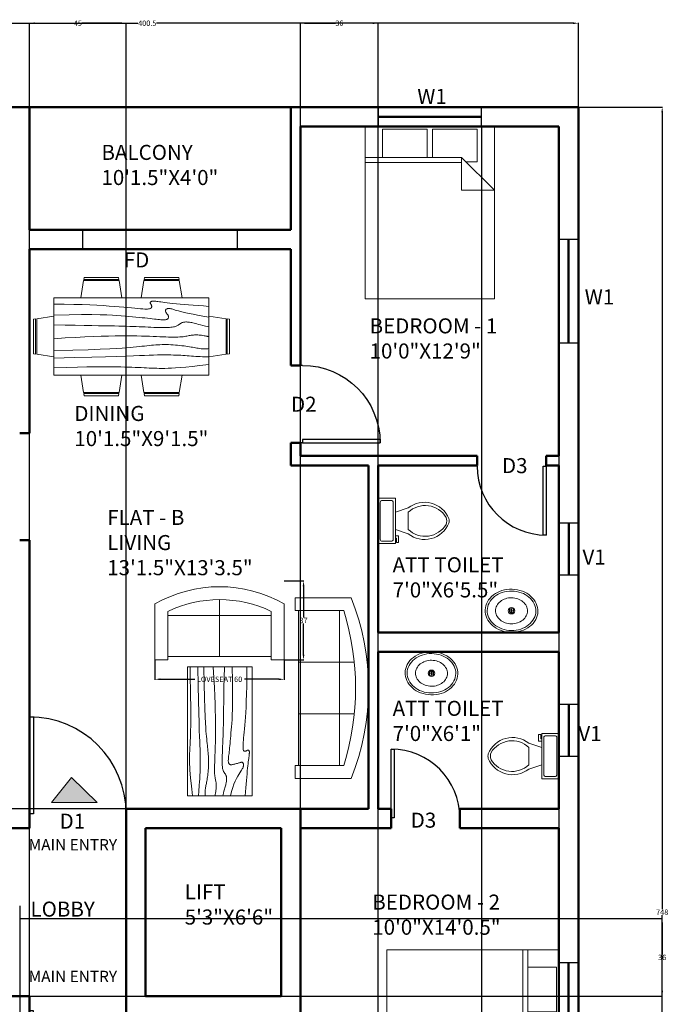
# Model space of a CAD drawing. Units: inches. Extents: x 227 to 711, y 218 to 1048.
# Tile 5 of 5: x 410 to 711, y 590 to 1048. Entities that reach past the tile are written whole.
import ezdxf

# ---------------------------------------------------------------- set-up
doc = ezdxf.new("R2010")
doc.units = ezdxf.units.IN
doc.header["$MEASUREMENT"] = 0
for name, color, linetype, lineweight in [('A-ANNO-DIMS', 2, 'Continuous', 18), ('A-ANNO-SYMB', 85, 'Continuous', 18), ('A-ANNO-TEXT', 70, 'Continuous', 18), ('A-AREA-IDEN', 70, 'Continuous', 25), ('A-FLOR-FIXT', 140, 'Continuous', 18), ('A-FURN', 8, 'Continuous', 18), ('A-WALL', 10, 'Continuous', 50), ('DOORS', 30, 'Continuous', 25), ('WINDOWS', 50, 'Continuous', 25)]:
    doc.layers.add(name, color=color, linetype=linetype, lineweight=lineweight)
doc.styles.get("Standard").update_dxf_attribs({"font": 'arial.ttf'})
doc.dimstyles.get("Standard").update_dxf_attribs({"dimtxt": 2.5, "dimasz": 2.5, "dimexe": 0.18, "dimexo": 0.0625, "dimgap": 0.09, "dimtad": 0, "dimtih": 1, "dimtoh": 1, "dimzin": 0, "dimdsep": 46, "dimlunit": 3, "dimtxsty": 'Standard', "dimcen": 0.09, "dimadec": 0, "dimazin": 0, "dimtfac": 1, "dimtofl": 0, "dimtmove": 0, "dimatfit": 3, "dimfxl": 1, "dimtolj": 1, "dimtzin": 0, "dimarcsym": 0})

# ---------------------------------------------------------------- blocks, each defined once
blk = doc.blocks.new('*U2')
for p, q in [((0, 0), (0, -6)), ((40, 0), (40, -6))]:
    blk.add_line(p, q)
blk.add_lwpolyline([(0, 0), (0, 40), (1.75, 40), (1.75, 0)], close=True)
blk.add_arc((0, 0), 40, 0, 90)
blk = doc.blocks.new('Bed - Queen')
for p, q in [((0, -80.00003), (0, 0)), ((0, 0), (59.99999, 0)), ((59.99999, 0), (59.99999, -80.00003)), ((7.99999, -1.2), (28.79998, -1.2)), ((7.99999, -14.4), (7.99999, -1.2)), ((28.79998, -1.2), (28.79998, -14.4)), ((31.19999, -1.2), (51.99999, -1.2)), ((31.19999, -14.4), (31.19999, -1.2)), ((51.99999, -1.2), (51.99999, -16.4)), ((0, -14.4), (44.8, -14.4)), ((44.8, -16.8), (0, -16.8)), ((59.99999, -29.6), (44.8, -14.4)), ((44.8, -14.4), (44.8, -29.6)), ((51.99999, -16.4), (46.79936, -16.4)), ((44.8, -29.6), (59.99999, -29.6)), ((59.99999, -80.00003), (0, -80.00003))]:
    blk.add_line(p, q)
blk = doc.blocks.new('Toilet - top')
for p, q in [((9.5, -6), (9.5, -2)), ((-10, -8.5), (-8, -8.5)), ((-10, -9.5), (-10, -8.5)), ((-8, -8.5), (-8, -8)), ((-7, -8), (-7, -9.5)), ((-4, -8), (-6, -14)), ((4, -8), (6, -14)), ((-7, -9.5), (-10, -9.5)), ((4, -14), (-4, -14))]:
    blk.add_line(p, q)
blk.add_lwpolyline([(10.5, -8), (10.5, 0), (-10.5, 0), (-10.5, -8)], close=True)
for points in [[(-9.5, -2), (-9.5, -6)], [(8.5, -1), (-8.5, -1)], [(-8.5, -7), (8.5, -7)]]:
    blk.add_lwpolyline(points)
for centre, radius, start, end in [((-8.62, -1.88), 0.884, 81.8699, 188.1301), ((8.62, -1.88), 0.884, 351.8699, 98.1301), ((-8.62, -6.12), 0.884, 171.8699, 278.1301), ((8.62, -6.12), 0.884, 261.8699, 8.1301), ((3.52, -21.58), 12.17, 141.4691, 247.9714), ((4.2, -21.82), 11.33, 136.3677, 238.9468), ((-3.52, -21.58), 12.17, 292.0284, 38.5307), ((-4.2, -21.82), 11.33, 301.053, 43.6321), ((0, -27.88), 4, 245.7318, 294.2682), ((0, -29), 4, 254.8605, 285.1395)]:
    blk.add_arc(centre, radius, start, end)
blk = doc.blocks.new('Sink - Oval top')
for p, q in [((-1, 0), (1, 0)), ((0, 1), (0, -1))]:
    blk.add_line(p, q)
for points in [[(-12.23, 0.39, 0.117634), (-11.46, -3.36, 0.104469), (-8.88, -6.8, 0.090016), (-5.08, -9.07, 0.08192), (-0.32, -10.02, 0.08192), (4.49, -9.38, 0.090016), (8.42, -7.36, 0.104469), (11.22, -4.09, 0.117634), (12.23, -0.39, 0.117634), (11.46, 3.36, 0.104469), (8.88, 6.8, 0.090016), (5.08, 9.07, 0.08192), (0.32, 10.02, 0.08192), (-4.49, 9.38, 0.090016), (-8.42, 7.36, 0.104469), (-11.22, 4.09, 0.117634)], [(-11.29, 0.16, 0.118622), (-10.52, -3.25, 0.104678), (-8.07, -6.36, 0.089562), (-4.54, -8.37, 0.081185), (-0.13, -9.15, 0.081185), (4.3, -8.49, 0.089562), (7.89, -6.58, 0.104678), (10.42, -3.55, 0.118622), (11.29, -0.16, 0.118622), (10.52, 3.25, 0.104678), (8.07, 6.36, 0.089562), (4.54, 8.37, 0.081185), (0.13, 9.15, 0.081185), (-4.3, 8.49, 0.089562), (-7.89, 6.58, 0.104678), (-10.42, 3.55, 0.118622)], [(-7.42, 0.08, 0.118283), (-6.91, -2.17, 0.104607), (-5.29, -4.21, 0.089718), (-2.97, -5.53, 0.081436), (-0.07, -6.04, 0.081436), (2.84, -5.59, 0.089718), (5.2, -4.33, 0.104607), (6.86, -2.32, 0.118283), (7.42, -0.08, 0.118283), (6.91, 2.17, 0.104607), (5.29, 4.21, 0.089718), (2.97, 5.53, 0.081436), (0.07, 6.04, 0.081436), (-2.84, 5.59, 0.089718), (-5.2, 4.33, 0.104607), (-6.86, 2.32, 0.118283)]]:
    blk.add_lwpolyline(points, format="xyb", close=True)
for radius in [1.5, 1]:
    blk.add_circle((0, 0), radius)
blk = doc.blocks.new('Sofa - Roundback 7 ft.')
for p, q in [((-12.00002, -32.4421), (-12.00003, -6.5971)), ((11.99997, -32.4421), (11.99998, -6.5971)), ((-36.000027, -34), (-36.000027, -11.4696)), ((-35.999844, -13.3819), (35.9998, -13.3819)), ((35.99998, -34), (35.99998, -11.4696)), ((-36.000027, -32.4421), (35.99998, -32.4421))]:
    blk.add_line(p, q)
for points in [[(-36.000027, -34), (-42.000027, -34), (-42.000027, -8)], [(41.99998, -8), (41.99998, -34), (35.99998, -34)]]:
    blk.add_lwpolyline(points)
for centre, radius, start, end in [((0, -114.25), 114.25, 68.43141, 111.5686), ((-0.00001, -127.1968), 121.1968, 72.72033, 107.2797)]:
    blk.add_arc(centre, radius, start, end)
blk = doc.blocks.new('Sofa - Roundback Loveseat 5 ft.')
for p, q in [((0, -32.44198), (0, -5.99998)), ((-24, -33.99998), (-24, -11.46958)), ((-23.9998, -13.38178), (23.99986, -13.38178)), ((24.00004, -33.99998), (24.00004, -11.46958)), ((-24, -32.44198), (24.00004, -32.44198))]:
    blk.add_line(p, q)
for points in [[(-24, -33.99998), (-30, -33.99998), (-30, -7.99998)], [(30.00004, -7.99998), (30.00004, -33.99998), (24.00004, -33.99998)]]:
    blk.add_lwpolyline(points)
for centre, radius, start, end in [((0, -60.24998), 60.24998, 60.13715, 119.8628), ((0, -61.38438), 55.38444, 64.32083, 115.6792)]:
    blk.add_arc(centre, radius, start, end)
blk = doc.blocks.new('Dining Set - 36 x 72 in.')
for p, q in [((-22, 27.5), (-22.1562, 26.50042)), ((-22, 27.5), (-6, 27.5)), ((-5.8437, 26.49966), (-6, 27.5)), ((6, 27.5), (5.8438, 26.50042)), ((6, 27.5), (22, 27.5)), ((22.1563, 26.49966), (22, 27.5)), ((-22.2343, 26.00059), (-23.4847, 17.99762)), ((-22.2304, 26), (-5.7608, 26)), ((-5.8416, 26.5), (-22.1534, 26.5)), ((-4.5152, 17.99762), (-5.7655, 25.99926)), ((5.7657, 26.00059), (4.5153, 17.99762)), ((5.7696, 26), (22.2392, 26)), ((22.1584, 26.5), (5.8466, 26.5)), ((23.4848, 17.99762), (22.2345, 25.99926)), ((36, 18), (-36, 18)), ((-36, 18), (-36, -18)), ((36, -18), (36, 18)), ((-44.0006, 8.23428), (-35.9976, 9.48474)), ((44.0006, 8.23428), (35.9976, 9.48474)), ((-45.5, 8), (-44.5004, 8.15617)), ((-45.5, 8), (-45.5, -8)), ((-44.5, -8.15843), (-44.5, 8.15338)), ((-44, 8.23041), (-44, -8.23915)), ((44, 8.23041), (44, -8.23915)), ((44.5, -8.15843), (44.5, 8.15338)), ((45.5, 8), (44.5005, 8.15617)), ((45.5, 8), (45.5, -8)), ((-44.4997, -8.15631), (-45.5, -8)), ((-35.9976, -9.48476), (-43.9993, -8.2345)), ((35.9976, -9.48476), (43.9993, -8.2345)), ((44.4997, -8.15631), (45.5, -8)), ((-36, -18), (36, -18)), ((-22.2343, -26.0006), (-23.4847, -17.99762)), ((-4.5152, -17.99762), (-5.7655, -25.99928)), ((5.7657, -26.0006), (4.5153, -17.99762)), ((23.4848, -17.99762), (22.2345, -25.99928)), ((-22.2304, -26), (-5.7608, -26)), ((-22, -27.5), (-22.1562, -26.50044)), ((-5.8416, -26.5), (-22.1534, -26.5)), ((-5.8437, -26.49967), (-6, -27.5)), ((5.7696, -26), (22.2392, -26)), ((6, -27.5), (5.8438, -26.50044)), ((22.1584, -26.5), (5.8466, -26.5)), ((22.1563, -26.49967), (22, -27.5)), ((-22, -27.5), (-6, -27.5)), ((6, -27.5), (22, -27.5))]:
    blk.add_line(p, q)
for points in [[(-36, 15), (-31.1772, 14.97754), (-26.8079, 14.91406), (-22.8538, 14.81543), (-19.276, 14.6875), (-16.0362, 14.53613), (-13.0957, 14.36718), (-10.4159, 14.18652), (-7.9583, 14), (-5.6904, 13.81315), (-3.6035, 13.63021), (-1.6954, 13.45508), (0.0365, 13.29166), (1.5945, 13.14388), (2.9811, 13.01562), (4.1988, 12.9108), (5.25, 12.83333), (6.1393, 12.78613), (6.8802, 12.76823), (7.4883, 12.77767), (7.9792, 12.8125), (8.3685, 12.87077), (8.6719, 12.95052), (8.9049, 13.0498), (9.0833, 13.16666), (9.2205, 13.29899), (9.3216, 13.44401), (9.3895, 13.59879), (9.4271, 13.76041), (9.4373, 13.92594), (9.4232, 14.09245), (9.3875, 14.257), (9.3333, 14.41666), (9.2638, 14.56917), (9.1836, 14.71484), (9.0975, 14.85465), (9.0104, 14.98958), (8.9272, 15.1206), (8.8529, 15.2487), (8.7922, 15.37483), (8.75, 15.5), (8.7305, 15.62467), (8.7344, 15.74739), (8.7617, 15.86621), (8.8125, 15.97916), (8.8867, 16.08431), (8.9844, 16.17968), (9.1055, 16.26334), (9.25, 16.33333), (9.4189, 16.38802), (9.6172, 16.42708), (9.8506, 16.45052), (10.125, 16.45833), (10.4463, 16.45052), (10.8203, 16.42708), (11.2529, 16.38802), (11.75, 16.33333), (12.3184, 16.26318), (12.9694, 16.17838), (13.7151, 16.07991), (14.5677, 15.96875), (15.5395, 15.84586), (16.6426, 15.71224), (17.8893, 15.56884), (19.2917, 15.41666), (20.859, 15.25667), (22.5879, 15.08984), (24.4721, 14.91715), (26.5052, 14.73958), (28.6809, 14.5581), (30.9929, 14.3737), (33.4347, 14.18733), (36, 14)], [(-36, 10), (-28.9766, 10.14274), (-23.1725, 10.20442), (-18.4241, 10.19775), (-14.5677, 10.13541), (-11.4399, 10.03011), (-8.877, 9.89453), (-6.7154, 9.74137), (-4.7917, 9.58333), (-2.9698, 9.43082), (-1.2246, 9.28515), (0.4415, 9.14534), (2.026, 9.01041), (3.5266, 8.87939), (4.9408, 8.7513), (6.266, 8.62516), (7.5, 8.5), (8.6411, 8.37549), (9.6914, 8.2539), (10.6538, 8.13818), (11.5312, 8.03125), (12.3267, 7.93603), (13.043, 7.85547), (13.6831, 7.79248), (14.25, 7.75), (14.7471, 7.7303), (15.1797, 7.73307), (15.5537, 7.75732), (15.875, 7.80208), (16.1494, 7.86637), (16.3828, 7.94922), (16.5811, 8.04964), (16.75, 8.16666), (16.8944, 8.29915), (17.0143, 8.44531), (17.1089, 8.60319), (17.1771, 8.77083), (17.218, 8.94629), (17.2305, 9.1276), (17.2137, 9.31282), (17.1667, 9.5), (17.0895, 9.6875), (16.987, 9.875), (16.8649, 10.0625), (16.7292, 10.25), (16.5856, 10.4375), (16.4401, 10.625), (16.2985, 10.8125), (16.1667, 11), (16.05, 11.18733), (15.9518, 11.3737), (15.8752, 11.5581), (15.8229, 11.73958), (15.798, 11.91715), (15.8034, 12.08984), (15.842, 12.25667), (15.9167, 12.41666), (16.0295, 12.56836), (16.1784, 12.70833), (16.3605, 12.83268), (16.5729, 12.9375), (16.8127, 13.01888), (17.0768, 13.07291), (17.3625, 13.0957), (17.6667, 13.08333), (17.9894, 13.03312), (18.3418, 12.94726), (18.7382, 12.82918), (19.1927, 12.68229), (19.7195, 12.51001), (20.3327, 12.31575), (21.0465, 12.10294), (21.875, 11.875), (22.8357, 11.63354), (23.959, 11.37304), (25.2786, 11.08618), (26.8282, 10.76562), (28.6414, 10.40405), (30.752, 9.99414), (33.1936, 9.52856), (36, 9)], [(-36, 5.5), (-30.7157, 5.3348), (-26.069, 5.20963), (-21.9946, 5.11767), (-18.4271, 5.05208), (-15.3009, 5.00602), (-12.5508, 4.97265), (-10.1112, 4.94515), (-7.9167, 4.91666), (-5.909, 4.88167), (-4.0586, 4.83984), (-2.3429, 4.79215), (-0.7396, 4.73958), (0.7739, 4.6831), (2.22, 4.6237), (3.6213, 4.56233), (5, 4.5), (6.373, 4.43782), (7.7344, 4.3776), (9.0723, 4.32129), (10.375, 4.27083), (11.6309, 4.22819), (12.8281, 4.19531), (13.9551, 4.17415), (15, 4.16666), (15.954, 4.17448), (16.819, 4.19791), (17.6001, 4.23698), (18.3021, 4.29166), (18.9299, 4.36198), (19.4883, 4.44791), (19.9823, 4.54948), (20.4167, 4.66666), (20.7969, 4.79899), (21.1302, 4.94401), (21.4245, 5.09879), (21.6875, 5.26041), (21.9271, 5.42594), (22.1511, 5.59245), (22.3672, 5.757), (22.5834, 5.91666), (22.8065, 6.06868), (23.0404, 6.21093), (23.2879, 6.34147), (23.5521, 6.45833), (23.8358, 6.55957), (24.142, 6.64323), (24.4735, 6.70735), (24.8334, 6.75), (25.2235, 6.76969), (25.642, 6.76692), (26.0858, 6.74267), (26.5521, 6.69791), (27.0379, 6.63362), (27.5404, 6.55078), (28.0565, 6.45036), (28.5834, 6.33333), (29.1242, 6.19987), (29.7071, 6.04687), (30.3661, 5.87044), (31.1354, 5.66666), (32.0493, 5.43164), (33.142, 5.16146), (34.4475, 4.85221), (36, 4.5)], [(-36, -1), (-30.7915, -0.6591), (-26.0195, -0.38216), (-21.6519, -0.16284), (-17.6563, 0.00521), (-14.0005, 0.12833), (-10.6523, 0.21289), (-7.5796, 0.26522), (-4.75, 0.29166), (-2.134, 0.29793), (0.2878, 0.28711), (2.5317, 0.26163), (4.6146, 0.22396), (6.5529, 0.17651), (8.3633, 0.12174), (10.0623, 0.06209), (11.6667, 0), (13.1899, -0.06201), (14.6341, -0.1211), (15.9982, -0.17432), (17.2813, -0.21875), (18.4823, -0.25147), (19.6003, -0.26953), (20.6343, -0.27002), (21.5834, -0.25), (22.4481, -0.20768), (23.2357, -0.14584), (23.9549, -0.06836), (24.6146, 0.02083), (25.2235, 0.11784), (25.7904, 0.21875), (26.3241, 0.31966), (26.8334, 0.41666), (27.3265, 0.50618), (27.8099, 0.58593), (28.2894, 0.65397), (28.7709, 0.70833), (29.2601, 0.74707), (29.763, 0.76823), (30.2855, 0.76985), (30.8334, 0.75), (31.4088, 0.70784), (31.9994, 0.64713), (32.589, 0.57275), (33.1615, 0.48958), (33.7008, 0.4025), (34.1908, 0.3164), (34.6153, 0.23616), (34.9584, 0.16666), (35.2099, 0.11165), (35.3848, 0.07031), (35.504, 0.04069), (35.5886, 0.02083), (35.6594, 0.00879), (35.7377, 0.0026), (35.8442, 0.00032), (36, 0)], [(-36, -6.5), (-27.1843, -6.31267), (-20.084, -6.1263), (-14.469, -5.9419), (-10.1094, -5.76042), (-6.7752, -5.58285), (-4.2363, -5.41016), (-2.2629, -5.24333), (-0.625, -5.08334), (0.8708, -4.93099), (2.2715, -4.78646), (3.5872, -4.64974), (4.8281, -4.52084), (6.0046, -4.39974), (7.127, -4.28646), (8.2053, -4.18099), (9.25, -4.08334), (10.2705, -3.99382), (11.2734, -3.91407), (12.2647, -3.84603), (13.25, -3.79167), (14.2354, -3.75293), (15.2266, -3.73177), (16.2295, -3.73015), (17.25, -3.75), (18.2912, -3.79248), (19.3451, -3.85547), (20.4009, -3.93604), (21.4479, -4.03125), (22.4754, -4.13819), (23.4727, -4.25391), (24.4289, -4.37549), (25.3334, -4.5), (26.1785, -4.62492), (26.9694, -4.74935), (27.7145, -4.87281), (28.4219, -4.99479), (29.1, -5.11483), (29.7572, -5.23242), (30.4016, -5.34709), (31.0417, -5.45834), (31.6837, -5.56437), (32.3262, -5.65821), (32.9658, -5.73153), (33.599, -5.77604), (34.2224, -5.78345), (34.8327, -5.74545), (35.4264, -5.65373), (36, -5.5)], [(-36, -10), (-26.4022, -9.81299), (-18.4675, -9.62891), (-11.9839, -9.45069), (-6.7396, -9.28125), (-2.5226, -9.12354), (0.8789, -8.98047), (3.6769, -8.85498), (6.0833, -8.75), (8.2767, -8.66765), (10.3021, -8.60677), (12.1712, -8.56543), (13.8958, -8.54167), (15.4876, -8.53353), (16.9583, -8.53907), (18.3197, -8.55632), (19.5834, -8.58334), (20.7616, -8.61841), (21.8685, -8.66081), (22.9188, -8.71004), (23.9271, -8.76563), (24.9081, -8.82707), (25.8763, -8.89388), (26.8465, -8.96558), (27.8334, -9.04167), (28.8474, -9.12118), (29.8828, -9.20117), (30.93, -9.27824), (31.9792, -9.34896), (33.0205, -9.40991), (34.0443, -9.45768), (35.0407, -9.48885), (36, -9.5)], [(-36, -14.5), (-30.0881, -14.33513), (-25.0332, -14.21224), (-20.7312, -14.12647), (-17.0781, -14.07292), (-13.97, -14.04671), (-11.3027, -14.04297), (-8.9724, -14.05681), (-6.875, -14.08334), (-4.9224, -14.11833), (-3.0905, -14.16016), (-1.3709, -14.20785), (0.2448, -14.26042), (1.7647, -14.3169), (3.1973, -14.3763), (4.5507, -14.43767), (5.8333, -14.5), (7.0554, -14.5621), (8.235, -14.62175), (9.3922, -14.67652), (10.5469, -14.72396), (11.7192, -14.76164), (12.929, -14.78711), (14.1965, -14.79794), (15.5417, -14.79167), (16.9933, -14.76424), (18.6152, -14.70508), (20.4804, -14.60197), (22.6615, -14.44271), (25.2312, -14.21509), (28.2624, -13.9069), (31.8277, -13.50594), (36, -13)]]:
    blk.add_lwpolyline(points)
blk = doc.blocks.new('Table - Rectangular Woodgrain 60 x 30 in.')
for p, q in [((0, 0), (0, -30)), ((60, 0), (0, 0)), ((60, -30), (60, 0)), ((0, -30), (60, -30))]:
    blk.add_line(p, q)
for points in [[(0, -2.4), (4.8155, -2.418), (9.0302, -2.4688), (12.709, -2.5477), (15.9167, -2.65), (18.7181, -2.7711), (21.1781, -2.9063), (23.3616, -3.0508), (25.3333, -3.2), (27.1477, -3.3495), (28.8172, -3.4958), (30.3437, -3.636), (31.7291, -3.7667), (32.9756, -3.8849), (34.0849, -3.9875), (35.059, -4.0714), (35.9, -4.1334), (36.6114, -4.1711), (37.2041, -4.1854), (37.6906, -4.1779), (38.0833, -4.15), (38.3948, -4.1034), (38.6375, -4.0396), (38.8239, -3.9602), (38.9666, -3.8667), (39.0764, -3.7608), (39.1573, -3.6448), (39.2116, -3.521), (39.2416, -3.3917), (39.2498, -3.2593), (39.2385, -3.1261), (39.21, -2.9944), (39.1666, -2.8667), (39.111, -2.7447), (39.0468, -2.6281), (38.978, -2.5163), (38.9083, -2.4083), (38.8418, -2.3035), (38.7823, -2.201), (38.7337, -2.1001), (38.7, -2), (38.6844, -1.9003), (38.6875, -1.8021), (38.7094, -1.707), (38.75, -1.6167), (38.8094, -1.5326), (38.8875, -1.4563), (38.9844, -1.3893), (39.1, -1.3333), (39.2351, -1.2896), (39.3937, -1.2583), (39.5804, -1.2396), (39.8, -1.2333), (40.057, -1.2396), (40.3562, -1.2583), (40.7023, -1.2896), (41.1, -1.3333), (41.5547, -1.3895), (42.0755, -1.4573), (42.6721, -1.5361), (43.3542, -1.625), (44.1316, -1.7233), (45.014, -1.8302), (46.0114, -1.9449), (47.1333, -2.0667), (48.3862, -2.1947), (49.7625, -2.3281), (51.2513, -2.4663), (52.8416, -2.6083), (54.5226, -2.7535), (56.2833, -2.9011), (58.1127, -3.0501), (60, -3.2)], [(0, -9.2), (6.5759, -9.0858), (11.9385, -9.0365), (16.2527, -9.0418), (19.6833, -9.0917), (22.3952, -9.1759), (24.5531, -9.2844), (26.322, -9.4069), (27.8666, -9.5333), (29.3241, -9.6553), (30.7203, -9.7719), (32.0532, -9.8837), (33.3208, -9.9917), (34.5213, -10.0965), (35.6526, -10.199), (36.7128, -10.2999), (37.7, -10.4), (38.6129, -10.4996), (39.4531, -10.5969), (40.223, -10.6895), (40.925, -10.775), (41.5613, -10.8512), (42.1344, -10.9156), (42.6465, -10.966), (43.1, -11), (43.4976, -11.0158), (43.8437, -11.0136), (44.143, -10.9942), (44.4, -10.9583), (44.6195, -10.9069), (44.8062, -10.8406), (44.9648, -10.7603), (45.1, -10.6667), (45.2155, -10.5598), (45.3114, -10.4365), (45.3871, -10.2929), (45.4416, -10.125), (45.4743, -9.929), (45.4844, -9.7011), (45.4709, -9.4371), (45.4333, -9.1333), (45.3716, -8.7883), (45.2896, -8.4104), (45.1919, -8.0107), (45.0833, -7.6), (44.9685, -7.1893), (44.8521, -6.7896), (44.7388, -6.4117), (44.6333, -6.0667), (44.54, -5.7628), (44.4614, -5.4979), (44.4001, -5.2675), (44.3583, -5.0667), (44.3384, -4.8909), (44.3427, -4.7354), (44.3736, -4.5956), (44.4333, -4.4667), (44.5236, -4.3453), (44.6427, -4.2333), (44.7884, -4.1339), (44.9583, -4.05), (45.1501, -3.9849), (45.3614, -3.9417), (45.59, -3.9234), (45.8333, -3.9333), (46.0915, -3.9749), (46.3734, -4.0531), (46.6906, -4.1736), (47.0542, -4.3417), (47.4756, -4.5629), (47.9661, -4.8427), (48.5372, -5.1866), (49.2, -5.6), (49.9676, -6.0844), (50.8594, -6.625), (51.8965, -7.2031), (53.1, -7.8), (54.491, -8.3969), (56.0906, -8.975), (57.9199, -9.5156), (60, -10)], [(0, -12.8), (5.1847, -12.9322), (9.6213, -13.0323), (13.3963, -13.1059), (16.5958, -13.1583), (19.3063, -13.1952), (21.614, -13.2219), (23.6054, -13.2439), (25.3666, -13.2667), (26.9728, -13.2947), (28.4531, -13.3281), (29.8256, -13.3663), (31.1083, -13.4083), (32.3191, -13.4535), (33.476, -13.501), (34.597, -13.5501), (35.7, -13.6), (36.7984, -13.6497), (37.8875, -13.6979), (38.9578, -13.743), (40, -13.7833), (41.0047, -13.8174), (41.9625, -13.8438), (42.864, -13.8607), (43.7, -13.8667), (44.4631, -13.8604), (45.1552, -13.8417), (45.7801, -13.8104), (46.3416, -13.7667), (46.8439, -13.7104), (47.2906, -13.6417), (47.6858, -13.5604), (48.0333, -13.4667), (48.3375, -13.3608), (48.6042, -13.2448), (48.8396, -13.121), (49.05, -12.9917), (49.2417, -12.8593), (49.4208, -12.7261), (49.5937, -12.5944), (49.7667, -12.4667), (49.9452, -12.3451), (50.1323, -12.2313), (50.3303, -12.1268), (50.5416, -12.0333), (50.7686, -11.9524), (51.0135, -11.8854), (51.2788, -11.8341), (51.5666, -11.8), (51.8785, -11.7843), (52.2116, -11.7865), (52.562, -11.8059), (52.926, -11.8417), (53.2998, -11.8931), (53.6795, -11.9594), (54.0614, -12.0397), (54.4416, -12.1333), (54.8223, -12.2401), (55.2293, -12.3625), (55.6942, -12.5037), (56.2489, -12.6667), (56.9251, -12.8547), (57.7545, -13.0708), (58.7689, -13.3182), (60, -13.6)], [(0, -18), (5.124, -17.7273), (9.6609, -17.5057), (13.6705, -17.3303), (17.2125, -17.1958), (20.3467, -17.0973), (23.1328, -17.0297), (25.6307, -16.9878), (27.9, -16.9667), (29.9928, -16.9617), (31.9302, -16.9703), (33.7254, -16.9907), (35.3917, -17.0208), (36.9423, -17.0588), (38.3906, -17.1026), (39.7499, -17.1503), (41.0333, -17.2), (42.2519, -17.2496), (43.4073, -17.2969), (44.4986, -17.3395), (45.525, -17.375), (46.4858, -17.4012), (47.3802, -17.4156), (48.2074, -17.416), (48.9667, -17.4), (49.6583, -17.3662), (50.2872, -17.3167), (50.8595, -17.2547), (51.3812, -17.1833), (51.8584, -17.1057), (52.2971, -17.025), (52.7034, -16.9443), (53.0833, -16.8667), (53.443, -16.7951), (53.789, -16.7313), (54.128, -16.6768), (54.4666, -16.6334), (54.8115, -16.6024), (55.1693, -16.5854), (55.5465, -16.5841), (55.95, -16.6), (56.3828, -16.6337), (56.8346, -16.6823), (57.2915, -16.7418), (57.7396, -16.8084), (58.165, -16.878), (58.5539, -16.9469), (58.8924, -17.0111), (59.1666, -17.0667), (59.3679, -17.1107), (59.5078, -17.1438), (59.6032, -17.1675), (59.6708, -17.1833), (59.7275, -17.193), (59.7901, -17.1979), (59.8753, -17.1998), (60, -17.2)], [(0, -22.4), (8.0098, -22.2501), (14.4094, -22.1011), (19.4168, -21.9535), (23.25, -21.8083), (26.1269, -21.6663), (28.2656, -21.5281), (29.884, -21.3947), (31.2, -21.2667), (32.3967, -21.1448), (33.5172, -21.0292), (34.5697, -20.9198), (35.5625, -20.8167), (36.5037, -20.7198), (37.4015, -20.6292), (38.2642, -20.5448), (39.1, -20.4667), (39.9164, -20.3951), (40.7187, -20.3313), (41.5117, -20.2768), (42.3, -20.2333), (43.0883, -20.2024), (43.8812, -20.1854), (44.6836, -20.1841), (45.5, -20.2), (46.3328, -20.234), (47.1747, -20.2844), (48.0163, -20.3488), (48.8479, -20.425), (49.66, -20.5106), (50.4429, -20.6031), (51.1872, -20.7004), (51.8833, -20.8), (52.5246, -20.8999), (53.1166, -20.9995), (53.6681, -21.0983), (54.1875, -21.1958), (54.6834, -21.2919), (55.1646, -21.3859), (55.6394, -21.4777), (56.1167, -21.5667), (56.6028, -21.6515), (57.0961, -21.7266), (57.5929, -21.7852), (58.0896, -21.8208), (58.5823, -21.8268), (59.0674, -21.7964), (59.5412, -21.723), (60, -21.6)], [(0, -25.2), (8.6355, -25.0504), (15.7026, -24.9031), (21.4049, -24.7606), (25.9458, -24.625), (29.529, -24.4988), (32.3578, -24.3844), (34.6359, -24.284), (36.5667, -24.2), (38.3213, -24.1341), (39.9417, -24.0854), (41.437, -24.0523), (42.8167, -24.0333), (44.0901, -24.0268), (45.2667, -24.0313), (46.3557, -24.0451), (47.3667, -24.0667), (48.309, -24.0947), (49.1928, -24.1287), (50.0284, -24.168), (50.826, -24.2125), (51.5959, -24.2617), (52.3483, -24.3151), (53.0935, -24.3725), (53.8417, -24.4334), (54.6009, -24.497), (55.3699, -24.561), (56.1454, -24.6226), (56.9239, -24.6792), (57.7021, -24.7279), (58.4764, -24.7662), (59.2435, -24.7911), (60, -24.8)], [(0, -28.8), (5.6867, -28.6681), (10.45, -28.5698), (14.407, -28.5012), (17.675, -28.4584), (20.3711, -28.4374), (22.6125, -28.4344), (24.5164, -28.4455), (26.2, -28.4667), (27.762, -28.4947), (29.2276, -28.5281), (30.6033, -28.5663), (31.8958, -28.6084), (33.1118, -28.6535), (34.2578, -28.7011), (35.3405, -28.7501), (36.3666, -28.8), (37.3443, -28.8497), (38.288, -28.8974), (39.2137, -28.9412), (40.1375, -28.9792), (41.0753, -29.0093), (42.0432, -29.0297), (43.0572, -29.0384), (44.1333, -29.0333), (45.2936, -29.0114), (46.5843, -28.9641), (48.0579, -28.8816), (49.7666, -28.7542), (51.7629, -28.5721), (54.0989, -28.3255), (56.8272, -28.0048), (60, -27.6)]]:
    blk.add_lwpolyline(points)
blk = doc.blocks.new('WIN-48IN')
for p, q in [((0, 4.75), (48, 4.75)), ((0, 4.25), (48, 4.25))]:
    blk.add_line(p, q)
blk.add_lwpolyline([(0, 0), (48, 0), (48, 9), (0, 9)], close=True)
blk = doc.blocks.new('VENT-V1-24IN')
for p, q in [((4.25, 24), (4.25, 0)), ((4.75, 24), (4.75, 0))]:
    blk.add_line(p, q)
blk.add_lwpolyline([(0, 24), (0, 0), (9, 0), (9, 24)], close=True)
blk = doc.blocks.new('DOOR-FD-72IN')
blk.add_lwpolyline([(0, 0), (72, 0), (72, 9), (0, 9)], close=True)
blk = doc.blocks.new('ENTRY-DIRECTION')
h = blk.add_hatch(color=256)
h.dxf.hatch_style = 1
h.paths.add_polyline_path([(21.25, 11.69), (0, 11.44), (12.11, 0)])
for p, q in [((21.25, 11.69), (0, 11.44)), ((0, 11.44), (12.11, 0)), ((12.11, 0), (21.25, 11.69))]:
    blk.add_line(p, q)
blk = doc.blocks.new('*D42')
at = {"layer": 'A-ANNO-DIMS', "color": 0, "lineweight": -2, "transparency": 16777216}
for p, q in [((472.84, 750.2), (472.84, 741.08)), ((532.84, 750.2), (532.84, 741.08)), ((475.34, 741.26), (491.31, 741.26)), ((530.34, 741.26), (514.36, 741.26))]:
    blk.add_line(p, q, dxfattribs=at)
at = {"layer": 'A-ANNO-DIMS', "color": 0, "transparency": 16777216}
for points in [[(475.34, 741.68), (475.34, 740.85), (472.84, 741.26)], [(530.34, 741.68), (530.34, 740.85), (532.84, 741.26)]]:
    blk.add_solid(points, dxfattribs=at)
at = {"layer": 'Defpoints', "color": 0, "transparency": 16777216}
for p in [(472.84, 750.26), (532.84, 750.26), (532.84, 741.26)]:
    blk.add_point(p, dxfattribs=at)
at = {"layer": 'A-ANNO-DIMS', "color": 0, "transparency": 16777216, "insert": (502.84, 741.26), "char_height": 2.5, "attachment_point": 5}
blk.add_mtext('\\A1;LOVESEAT 60', dxfattribs=at)
blk = doc.blocks.new('*D43')
at = {"layer": 'A-ANNO-DIMS', "color": 0, "lineweight": -2, "transparency": 16777216}
for p, q in [((532.9, 786.93), (542.02, 786.93)), ((541.84, 784.43), (541.84, 769.96)), ((541.84, 752.76), (541.84, 767.23)), ((532.9, 750.26), (542.02, 750.26))]:
    blk.add_line(p, q, dxfattribs=at)
at = {"layer": 'A-ANNO-DIMS', "color": 0, "transparency": 16777216}
for points in [[(541.42, 784.43), (542.25, 784.43), (541.84, 786.93)], [(541.42, 752.76), (542.25, 752.76), (541.84, 750.26)]]:
    blk.add_solid(points, dxfattribs=at)
at = {"layer": 'Defpoints', "color": 0, "transparency": 16777216}
for p in [(532.84, 786.93), (541.84, 786.93), (532.84, 750.26)]:
    blk.add_point(p, dxfattribs=at)
at = {"layer": 'A-ANNO-DIMS', "color": 0, "transparency": 16777216, "insert": (541.84, 768.6), "char_height": 2.5, "attachment_point": 5}
blk.add_mtext('\\A1;37', dxfattribs=at)
blk = doc.blocks.new('*D44')
at = {"layer": 'A-ANNO-DIMS', "color": 0, "lineweight": -2, "transparency": 16777216}
for p, q in [((268.99, 1007.13), (268.99, 1046.2)), ((271.49, 1046.02), (464.87, 1046.02)), ((666.99, 1046.02), (473.61, 1046.02)), ((669.49, 1007.13), (669.49, 1046.2))]:
    blk.add_line(p, q, dxfattribs=at)
at = {"layer": 'A-ANNO-DIMS', "color": 0, "transparency": 16777216}
for points in [[(271.49, 1046.43), (271.49, 1045.6), (268.99, 1046.02)], [(666.99, 1046.43), (666.99, 1045.6), (669.49, 1046.02)]]:
    blk.add_solid(points, dxfattribs=at)
at = {"layer": 'Defpoints', "color": 0, "transparency": 16777216}
for p in [(669.49, 1046.02), (268.99, 1007.07), (669.49, 1007.07)]:
    blk.add_point(p, dxfattribs=at)
at = {"layer": 'A-ANNO-DIMS', "color": 0, "transparency": 16777216, "insert": (469.24, 1046.02), "char_height": 2.5, "attachment_point": 5}
blk.add_mtext('\\A1;400.5', dxfattribs=at)
blk = doc.blocks.new('*D45')
at = {"layer": 'A-ANNO-DIMS', "color": 0, "lineweight": -2, "transparency": 16777216}
for p, q in [((669.55, 1007.07), (708.62, 1007.07)), ((708.44, 1004.57), (708.44, 634.43)), ((708.44, 261.57), (708.44, 631.7)), ((669.55, 259.07), (708.62, 259.07))]:
    blk.add_line(p, q, dxfattribs=at)
at = {"layer": 'A-ANNO-DIMS', "color": 0, "transparency": 16777216}
for points in [[(708.02, 1004.57), (708.86, 1004.57), (708.44, 1007.07)], [(708.02, 261.57), (708.86, 261.57), (708.44, 259.07)]]:
    blk.add_solid(points, dxfattribs=at)
at = {"layer": 'Defpoints', "color": 0, "transparency": 16777216}
for p in [(669.49, 1007.07), (708.44, 1007.07), (669.49, 259.07)]:
    blk.add_point(p, dxfattribs=at)
at = {"layer": 'A-ANNO-DIMS', "color": 0, "transparency": 16777216, "insert": (708.44, 633.07), "char_height": 2.5, "attachment_point": 5}
blk.add_mtext('\\A1;748', dxfattribs=at)
blk = doc.blocks.new('*D51')
at = {"layer": 'A-ANNO-DIMS', "color": 0, "lineweight": -2, "transparency": 16777216}
for p, q in [((268.93, 1007.07), (229.86, 1007.07)), ((230.04, 1004.57), (230.04, 845.43)), ((230.04, 683.57), (230.04, 842.7)), ((459.43, 681.07), (229.86, 681.07))]:
    blk.add_line(p, q, dxfattribs=at)
at = {"layer": 'A-ANNO-DIMS', "color": 0, "transparency": 16777216}
for points in [[(229.62, 1004.57), (230.46, 1004.57), (230.04, 1007.07)], [(229.62, 683.57), (230.46, 683.57), (230.04, 681.07)]]:
    blk.add_solid(points, dxfattribs=at)
at = {"layer": 'Defpoints', "color": 0, "transparency": 16777216}
for p in [(230.04, 1007.07), (268.99, 1007.07), (459.49, 681.07)]:
    blk.add_point(p, dxfattribs=at)
at = {"layer": 'A-ANNO-DIMS', "color": 0, "transparency": 16777216, "insert": (230.04, 844.07), "char_height": 2.5, "attachment_point": 5}
blk.add_mtext('\\A1;326', dxfattribs=at)
blk = doc.blocks.new('*D53')
at = {"layer": 'A-ANNO-DIMS', "color": 0, "lineweight": -2, "transparency": 16777216}
for p, q in [((414.49, 585.13), (414.49, 1046.2)), ((416.99, 1046.02), (435.05, 1046.02)), ((456.99, 1046.02), (438.93, 1046.02)), ((459.49, 585.13), (459.49, 1046.2))]:
    blk.add_line(p, q, dxfattribs=at)
at = {"layer": 'A-ANNO-DIMS', "color": 0, "transparency": 16777216}
for points in [[(416.99, 1046.43), (416.99, 1045.6), (414.49, 1046.02)], [(456.99, 1046.43), (456.99, 1045.6), (459.49, 1046.02)]]:
    blk.add_solid(points, dxfattribs=at)
at = {"layer": 'Defpoints', "color": 0, "transparency": 16777216}
for p in [(459.49, 1046.02), (414.49, 585.07), (459.49, 585.07)]:
    blk.add_point(p, dxfattribs=at)
at = {"layer": 'A-ANNO-DIMS', "color": 0, "transparency": 16777216, "insert": (436.99, 1046.02), "char_height": 2.5, "attachment_point": 5}
blk.add_mtext('\\A1;45', dxfattribs=at)
blk = doc.blocks.new('*D56')
at = {"layer": 'A-ANNO-DIMS', "color": 0, "lineweight": -2, "transparency": 16777216}
for p, q in [((540.49, 493.63), (540.49, 1046.2)), ((542.99, 1046.02), (556.61, 1046.02)), ((573.99, 1046.02), (560.37, 1046.02)), ((576.49, 493.03), (576.49, 1046.2))]:
    blk.add_line(p, q, dxfattribs=at)
at = {"layer": 'A-ANNO-DIMS', "color": 0, "transparency": 16777216}
for points in [[(542.99, 1046.43), (542.99, 1045.6), (540.49, 1046.02)], [(573.99, 1046.43), (573.99, 1045.6), (576.49, 1046.02)]]:
    blk.add_solid(points, dxfattribs=at)
at = {"layer": 'Defpoints', "color": 0, "transparency": 16777216}
for p in [(576.49, 1046.02), (540.49, 493.57), (576.49, 492.97)]:
    blk.add_point(p, dxfattribs=at)
at = {"layer": 'A-ANNO-DIMS', "color": 0, "transparency": 16777216, "insert": (558.49, 1046.02), "char_height": 2.5, "attachment_point": 5}
blk.add_mtext('\\A1;36', dxfattribs=at)
blk = doc.blocks.new('*D59')
at = {"layer": 'A-ANNO-DIMS', "color": 0, "lineweight": -2, "transparency": 16777216}
for p, q in [((410.05, 630.07), (708.62, 630.07)), ((708.44, 627.57), (708.44, 613.43)), ((708.44, 596.57), (708.44, 610.7)), ((410.05, 594.07), (708.62, 594.07))]:
    blk.add_line(p, q, dxfattribs=at)
at = {"layer": 'A-ANNO-DIMS', "color": 0, "transparency": 16777216}
for points in [[(708.02, 627.57), (708.86, 627.57), (708.44, 630.07)], [(708.02, 596.57), (708.86, 596.57), (708.44, 594.07)]]:
    blk.add_solid(points, dxfattribs=at)
at = {"layer": 'Defpoints', "color": 0, "transparency": 16777216}
for p in [(409.99, 630.07), (708.44, 630.07), (409.99, 594.07)]:
    blk.add_point(p, dxfattribs=at)
at = {"layer": 'A-ANNO-DIMS', "color": 0, "transparency": 16777216, "insert": (708.44, 612.07), "char_height": 2.5, "attachment_point": 5}
blk.add_mtext('\\A1;36', dxfattribs=at)
blk = doc.blocks.new('*D60')
at = {"layer": 'A-ANNO-DIMS', "color": 0, "lineweight": -2, "transparency": 16777216}
for p, q in [((459.49, 681), (459.49, 219.94)), ((409.99, 636), (409.99, 219.94)), ((412.49, 220.12), (431.34, 220.12)), ((456.99, 220.12), (438.14, 220.12))]:
    blk.add_line(p, q, dxfattribs=at)
at = {"layer": 'A-ANNO-DIMS', "color": 0, "transparency": 16777216}
for points in [[(412.49, 220.53), (412.49, 219.7), (409.99, 220.12)], [(456.99, 220.53), (456.99, 219.7), (459.49, 220.12)]]:
    blk.add_solid(points, dxfattribs=at)
at = {"layer": 'Defpoints', "color": 0, "transparency": 16777216}
for p in [(459.49, 681.07), (409.99, 636.07), (459.49, 220.12)]:
    blk.add_point(p, dxfattribs=at)
at = {"layer": 'A-ANNO-DIMS', "color": 0, "transparency": 16777216, "insert": (434.74, 220.12), "char_height": 2.5, "attachment_point": 5}
blk.add_mtext('\\A1;49.5', dxfattribs=at)
blk = doc.blocks.new('*D62')
at = {"layer": 'A-ANNO-DIMS', "color": 0, "lineweight": -2, "transparency": 16777216}
for p, q in [((624.49, 998), (624.49, 219.94)), ((660.49, 998), (660.49, 219.94)), ((626.99, 220.12), (640.61, 220.12)), ((657.99, 220.12), (644.37, 220.12))]:
    blk.add_line(p, q, dxfattribs=at)
at = {"layer": 'A-ANNO-DIMS', "color": 0, "transparency": 16777216}
for points in [[(626.99, 220.53), (626.99, 219.7), (624.49, 220.12)], [(657.99, 220.53), (657.99, 219.7), (660.49, 220.12)]]:
    blk.add_solid(points, dxfattribs=at)
at = {"layer": 'Defpoints', "color": 0, "transparency": 16777216}
for p in [(624.49, 998.07), (660.49, 998.07), (660.49, 220.12)]:
    blk.add_point(p, dxfattribs=at)
at = {"layer": 'A-ANNO-DIMS', "color": 0, "transparency": 16777216, "insert": (642.49, 220.12), "char_height": 2.5, "attachment_point": 5}
blk.add_mtext('\\A1;36', dxfattribs=at)

msp = doc.modelspace()

# ---------------------------------------------------------------- linework, layer by layer
at = {"layer": 'A-WALL'}
for p, q in [((414.49, 1007.065), (414.49, 950.065)), ((414.49, 1007.065), (535.99, 1007.065)), ((535.99, 1007.065), (535.99, 950.065)), ((660.49, 998.065), (540.49, 998.065)), ((540.49, 998.065), (540.49, 887.065)), ((660.49, 845.065), (660.49, 998.065)), ((535.99, 950.065), (414.49, 950.065)), ((535.99, 941.065), (414.49, 941.065)), ((414.49, 941.065), (414.49, 855.565)), ((535.99, 941.065), (535.99, 887.065)), ((535.99, 887.065), (540.49, 887.065)), ((409.99, 855.565), (414.49, 855.565)), ((535.99, 851.065), (540.49, 851.065)), ((535.99, 851.065), (535.99, 840.565)), ((540.49, 851.065), (540.49, 845.065)), ((622.49, 845.065), (540.49, 845.065)), ((622.49, 845.065), (622.49, 840.565)), ((660.49, 845.065), (654.49, 845.065)), ((654.49, 845.065), (654.49, 840.565)), ((571.99, 840.565), (535.99, 840.565)), ((571.99, 763.065), (571.99, 840.565)), ((576.49, 763.065), (576.49, 840.565)), ((622.49, 840.565), (576.49, 840.565)), ((660.49, 840.565), (654.49, 840.565)), ((660.49, 763.065), (660.49, 840.565)), ((409.99, 805.861), (414.49, 805.861)), ((414.49, 805.861), (414.49, 672.065)), ((571.99, 681.065), (571.99, 763.065)), ((660.49, 763.065), (576.49, 763.065)), ((660.49, 754.065), (576.49, 754.065)), ((576.49, 681.065), (576.49, 754.065)), ((660.49, 681.065), (660.49, 754.065)), ((414.49, 681.065), (414.49, 672.065)), ((571.99, 681.065), (459.49, 681.065)), ((582.49, 681.065), (576.49, 681.065)), ((582.49, 681.065), (582.49, 672.065)), ((660.49, 681.065), (614.49, 681.065)), ((614.49, 681.065), (614.49, 672.065)), ((414.49, 672.065), (277.99, 672.065)), ((531.49, 672.065), (468.49, 672.065)), ((571.99, 672.065), (540.49, 672.065)), ((582.49, 672.065), (571.99, 672.065)), ((660.49, 672.065), (614.49, 672.065)), ((660.49, 499.065), (660.49, 672.065)), ((414.49, 594.065), (277.99, 594.065)), ((414.49, 594.065), (414.49, 446.565)), ((414.49, 594.065), (414.49, 585.065)), ((531.49, 594.065), (468.49, 594.065))]:
    msp.add_line(p, q, dxfattribs=at)
for points in [[(414.49, 1007.065), (268.99, 1007.065), (268.99, 259.065), (414.49, 259.065)], [(535.99, 259.065), (669.49, 259.065), (669.49, 1007.065), (535.99, 1007.065)], [(459.49, 681.226), (459.49, 652.565), (459.49, 585.065)], [(468.49, 681.226), (468.49, 681.065)], [(531.49, 681.226), (531.49, 681.065)], [(540.49, 681.226), (540.49, 652.565), (540.49, 585.065)], [(468.49, 672.065), (468.49, 652.565), (468.49, 594.065)], [(531.49, 672.065), (531.49, 652.565), (531.49, 594.065)]]:
    msp.add_lwpolyline(points, dxfattribs=at)

# ---------------------------------------------------------------- block references
at = {"layer": 'A-ANNO-SYMB', "rotation": 179.3231801931449}
msp.add_blockref('ENTRY-DIRECTION', (446.184, 695.442), dxfattribs=at)
at = {"layer": 'A-FLOR-FIXT'}
for p, rotation in [((576.49, 814.845), 89.99999999999756), ((660.49, 705.565), 270)]:
    msp.add_blockref('Toilet - top', p, dxfattribs=dict(at, rotation=rotation))
for p in [(638.457, 773.089), (601.264, 744.049)]:
    msp.add_blockref('Sink - Oval top', p, dxfattribs=at)
at = {"layer": 'A-FURN'}
for name, p in [('Bed - Queen', (570.49, 998.065)), ('Dining Set - 36 x 72 in.', (461.903, 900.473)), ('Sofa - Roundback Loveseat 5 ft.', (502.835, 784.262))]:
    msp.add_blockref(name, p, dxfattribs=at)
at = {"layer": 'A-FURN', "rotation": 270}
for name, p in [('Sofa - Roundback 7 ft.', (571.99, 737.155)), ('Table - Rectangular Woodgrain 60 x 30 in.', (517.91, 747.068)), ('Bed - Queen', (660.49, 615.565))]:
    msp.add_blockref(name, p, dxfattribs=at)
at = {"layer": 'DOORS'}
msp.add_blockref('DOOR-FD-72IN', (439.24, 941.065), dxfattribs=at)
for p, xscale, yscale, zscale, rotation in [((541.39, 851.065), -0.9000000000000028, 0.9000000000000028, 0.9000000000000028, 270), ((654.49, 840.265), 0.8, 0.8, 0.8, 180), ((414.49, 587.314), -1.12510570773799, 1.12510570773799, 1.12510570773799, 180)]:
    msp.add_blockref('*U2', p, dxfattribs=dict(at, xscale=xscale, yscale=yscale, zscale=zscale, rotation=rotation))
for p, xscale, yscale, zscale in [((414.49, 678.815), 1.125000000000002, 1.125000000000002, 1.125000000000002), ((582.49, 676.865), 0.8, 0.8, 0.8)]:
    msp.add_blockref('*U2', p, dxfattribs=dict(at, xscale=xscale, yscale=yscale, zscale=zscale))
at = {"layer": 'WINDOWS'}
for name, p in [('WIN-48IN', (576.49, 998.065)), ('VENT-V1-24IN', (660.49, 789.815)), ('VENT-V1-24IN', (660.49, 705.565))]:
    msp.add_blockref(name, p, dxfattribs=at)
at = {"layer": 'WINDOWS', "rotation": 89.99999999999979}
for p in [(669.49, 897.565), (669.49, 561.565)]:
    msp.add_blockref('WIN-48IN', p, dxfattribs=at)

# ---------------------------------------------------------------- texts
at = {"layer": 'A-ANNO-TEXT', "attachment_point": 1}
for s, width, gutter_width, insert, char_height in [('W1', 74.58955, 1, (594.687, 1015.524), 7), ('FD', 74.58955, 1, (458.354, 939.559), 7), ('W1', 74.58955, 1, (672.452, 922.376), 7), ('D2', 74.58955, 1, (536.027, 872.533), 7), ('D3', 74.58955, 1, (634.015, 844.011), 7), ('V1', 74.58955, 1, (671.423, 801.531), 7), ('V1', 74.58955, 1, (669.49, 719.534), 7), ('D1', 74.58955, 1, (428.526, 678.86), 7), ('D3', 74.58955, 1, (591.609, 679.318), 7), ('MAIN ENTRY', 55.87031, 0.749, (414.171, 667.025), 5.2433), ('MAIN ENTRY', 55.87031, 0.749, (414.171, 605.854), 5.2433)]:
    msp.add_mtext_dynamic_manual_height_columns(s, width=width, gutter_width=gutter_width, heights=[0], dxfattribs=dict(at, insert=insert, char_height=char_height))
at = {"layer": 'A-AREA-IDEN', "char_height": 7, "attachment_point": 1}
for s, insert in [('BALCONY\\P10\'1.5"X4\'0"', (447.963, 989.517)), ('BEDROOM - 1\\P10\'0"X12\'9"', (572.519, 908.926)), ('DINING\\P10\'1.5"X9\'1.5"', (435.381, 868.242)), ('FLAT - B\\PLIVING\\P13\'1.5"X13\'3.5"', (450.647, 819.935)), ('ATT TOILET\\P7\'0"X6\'5.5"', (583.228, 797.948)), ('ATT TOILET\\P7\'0"X6\'1"', (583.228, 731.262)), ('LIFT\\P5\'3"X6\'6"', (486.646, 645.988)), ('BEDROOM - 2\\P10\'0"X14\'0.5"', (573.765, 641.264)), ('LOBBY', (414.997, 637.994))]:
    msp.add_mtext_dynamic_manual_height_columns(s, width=74.58955, gutter_width=1, heights=[0], dxfattribs=dict(at, insert=insert))

# ---------------------------------------------------------------- dimensions: what is measured, and where the dimension line sits
at = {"layer": 'A-ANNO-DIMS'}
for base, p1, p2, override, picture, middle in [((669.49, 1046.015), (268.99, 1007.065), (669.49, 1007.065), {"dimdec": 1, "dimlfac": 1, "dimrnd": 0, "dimzin": 0, "dimdsep": 46, "dimlunit": 2}, '*D44', (469.24, 1046.015)), ((459.49, 1046.015), (414.49, 585.065), (459.49, 585.065), {"dimdec": 0, "dimlfac": 1, "dimrnd": 0, "dimzin": 0, "dimdsep": 46, "dimlunit": 2}, '*D53', (436.99, 1046.015)), ((576.49, 1046.015), (540.49, 493.572), (576.49, 492.972), {"dimdec": 0, "dimlfac": 1, "dimrnd": 0, "dimzin": 0, "dimdsep": 46, "dimlunit": 2}, '*D56', (558.49, 1046.015)), ((660.49, 220.115), (624.49, 998.065), (660.49, 998.065), {"dimdec": 0, "dimlfac": 1, "dimrnd": 0, "dimzin": 0, "dimdsep": 46, "dimlunit": 2}, '*D62', (642.49, 220.115)), ((459.49, 220.115), (409.99, 636.065), (459.49, 681.065), {"dimdec": 1, "dimlfac": 1, "dimrnd": 0, "dimzin": 0, "dimdsep": 46, "dimlunit": 2}, '*D60', (434.74, 220.115))]:
    dim = msp.add_linear_dim(base=base, p1=p1, p2=p2, dimstyle='Standard', override=override, dxfattribs=at)
    dim.commit()
    dim.dimension.update_dxf_attribs({"geometry": picture, "text_midpoint": middle})
for base, p1, p2, picture, middle in [((230.04, 1007.065), (459.49, 681.065), (268.99, 1007.065), '*D51', (230.04, 844.065)), ((708.44, 1007.065), (669.49, 259.065), (669.49, 1007.065), '*D45', (708.44, 633.065)), ((541.835, 786.929), (532.835, 750.262), (532.835, 786.929), '*D43', (541.835, 768.596)), ((708.44, 630.065), (409.99, 594.065), (409.99, 630.065), '*D59', (708.44, 612.065))]:
    dim = msp.add_linear_dim(base=base, p1=p1, p2=p2, angle=90, dimstyle='Standard', override={"dimdec": 0, "dimlfac": 1, "dimrnd": 0, "dimzin": 0, "dimdsep": 46, "dimlunit": 2}, dxfattribs=at)
    dim.commit()
    dim.dimension.update_dxf_attribs({"geometry": picture, "text_midpoint": middle})
dim = msp.add_linear_dim(base=(532.835, 741.262), p1=(472.835, 750.262), p2=(532.835, 750.262), text='LOVESEAT <>', dimstyle='Standard', override={"dimdec": 0, "dimlfac": 1, "dimrnd": 0, "dimzin": 0, "dimdsep": 46, "dimlunit": 2}, dxfattribs=at)
dim.commit()
dim.dimension.update_dxf_attribs({"geometry": '*D42', "text_midpoint": (502.835, 741.262)})

doc.saveas('drawing.dxf')
